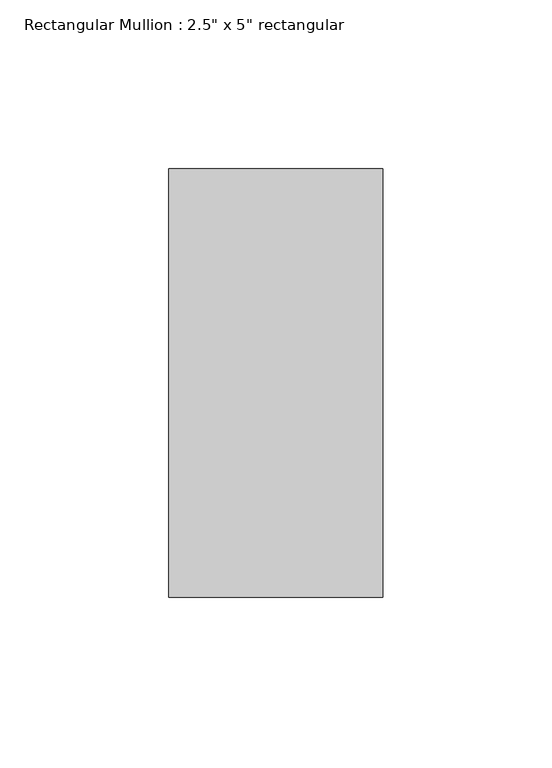
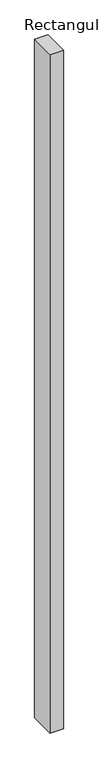
"""IFC4 building model written with IfcOpenShell, lengths in millimetres: member geometry."""

from ifc_helpers import new_model, si_unit, frame, origin, place, context, project, spatial, polyline, outline, extrude, source, transform, mapped, element, save


def member_6a95fd14(model_context):
    return source(origin(), model_context, "Body", "SweptSolid", [
        extrude(outline(polyline([(0.0, 63.5), (0.0, -63.5), (-63.5, -63.5), (-63.5, 63.5), (0.0, 63.5)])), frame((0.0, 0.0, -3431.8506278), z_axis=(0.0, 0.0, 1.0), x_axis=(1.0, 0.0, 0.0)), (0.0, 0.0, 1.0), 3431.8506278),
    ])


if __name__ == "__main__":
    model = new_model("IFC4")
    model_context = context("Model", 3, world=origin())
    ifc_project = project(units=[si_unit("LENGTHUNIT", "METRE", prefix="MILLI")], contexts=[model_context])
    site = spatial("IfcSite", under=ifc_project)
    building = spatial("IfcBuilding", under=site)
    placement = place(None, origin())
    member_shape = member_6a95fd14(model_context)
    element("IfcMember", 1, ObjectType="Rectangular Mullion : 2.5\" x 5\" rectangular", at=placement, inside=building, context=model_context, shape_type="MappedRepresentation", body=[
        mapped(member_shape, transform((0.0, 0.0, 0.0), x_axis=(1.0, 0.0, 0.0), y_axis=(0.0, 1.0, 0.0), z_axis=(0.0, 0.0, 1.0))),
    ])
    save(model, "model.ifc")

# Revit data of these elements
# Type "Rectangular Mullion : 2.5\" x 5\" rectangular"
#   built-in parameter 1007304 = 0.416667 (stored number, unit not read)
#   built-in parameter 1007301 = 0.104167 (stored number, unit not read)
#   built-in parameter 1007300 = 0.104167 (stored number, unit not read)
# Element 1 (IfcMember, "Rectangular Mullion : 2.5\" x 5\" rectangular")
#   Materials on its faces: "Iron, Ductile"
# Materials
#   "Iron, Ductile": class "Metal", colour RGB 0 0 0, transparency 0, Description = "Ductile cast iron", Cost = 0
